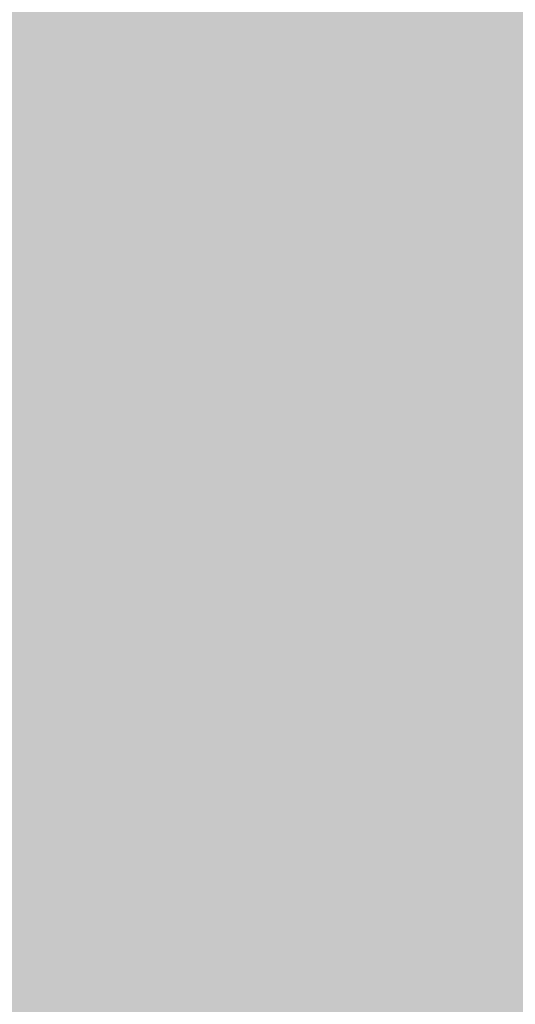
# Model space of a CAD drawing. Units: inches. Extents: x 2083 to 3317, y 1141 to 2115.
# Tile 165 of 256: x 3126.958245 to 3126.959398, y 1263.263648 to 1263.265937. Entities that reach past the tile are written whole.
import ezdxf

# ---------------------------------------------------------------- set-up
doc = ezdxf.new("R2010")
doc.units = ezdxf.units.IN
doc.layers.add('A-WALL-PATT', color=251, linetype='Continuous', lineweight=13, true_color=0x636466)

msp = doc.modelspace()

# ---------------------------------------------------------------- hatches: boundary and pattern name
at = {"layer": 'A-WALL-PATT'}
h = msp.add_hatch(color=256, dxfattribs=at)
h.dxf.hatch_style = 1
h.paths.add_polyline_path([(3126.9597832, 2020.7613601), (2748.9597832, 2020.7613601), (2604.9597832, 2020.7613601), (2226.9597832, 2020.7613601), (2226.9597832, 1702.7613601), (2466.9597832, 1702.7613601), (2466.9597832, 1582.7613601), (2418.9597832, 1582.7613601), (2418.9597832, 1477.7613601), (2226.9597832, 1477.7613601), (2226.9597832, 1263.2613601), (2544.9597832, 1263.2613601), (2544.9597832, 1411.7613601), (2604.9597832, 1411.7613601), (2685.9597832, 1411.7613601), (2685.9597832, 1420.7613601), (2604.9597832, 1420.7613601), (2604.9597832, 1573.7613601), (2604.9597832, 1702.7613601), (2604.9597832, 2011.7613601), (2748.9597832, 2011.7613601), (2748.9597832, 1702.7613601), (2862.9597832, 1702.7613601), (2862.9597832, 1621.7613601), (2871.9597832, 1621.7613601), (2871.9597832, 1702.7613601), (2883.9597832, 1702.7613601), (2883.9597832, 1706.9394595, -0.026459), (2883.9597832, 1711.7613601), (2757.9597832, 1711.7613601), (2757.9597832, 1807.7613601), (2787.9597832, 1807.7613601), (2787.9597832, 1812.2613601), (2757.9597832, 1812.2613601), (2757.9597832, 2011.7613601), (2877.9597832, 2011.7613601), (2877.9597832, 1812.2613601), (2847.9597832, 1812.2613601), (2847.9597832, 1807.7613601), (2889.8357425, 1807.7613601), (2889.8357425, 1812.2613601), (2882.4597832, 1812.2613601), (2882.4597832, 2011.7613601), (3117.9597832, 2011.7613601), (3117.9597832, 1812.2613601), (2937.8357425, 1812.2613601), (2937.8357425, 1807.7613601), (2995.7097832, 1807.7613601), (2995.7097832, 1796.1176655), (3000.2097832, 1796.1176655), (3000.2097832, 1807.7613601), (3117.9597832, 1807.7613601), (3117.9597832, 1711.7613601), (3000.2097832, 1711.7613601), (3000.2097832, 1760.1176655), (2998.5727047, 1760.1176655, -0.020711), (2995.7097832, 1760.1176655), (2995.7097832, 1711.7613601), (2931.9597832, 1711.7613601), (2931.9597832, 1702.7613601), (3126.9597832, 1702.7613601)])
h.paths.add_polyline_path([(2471.4597832, 2011.7613601), (2471.4597832, 1810.0113601), (2462.7169357, 1810.0113601), (2462.7169357, 1805.5113601), (2505.9597832, 1805.5113601), (2505.9597832, 1810.0113601), (2475.9597832, 1810.0113601), (2475.9597832, 2011.7613601), (2595.9597832, 2011.7613601), (2595.9597832, 1810.0113601), (2565.9597832, 1810.0113601), (2565.9597832, 1805.5113601), (2595.9597832, 1805.5113601), (2595.9597832, 1711.7613601), (2235.9597832, 1711.7613601), (2235.9597832, 1805.5113601), (2353.7097832, 1805.5113601), (2353.7097832, 1796.0541624), (2358.2097832, 1796.0541624), (2358.2097832, 1805.5113601), (2414.7169357, 1805.5113601), (2414.7169357, 1810.0113601), (2235.9597832, 1810.0113601), (2235.9597832, 2011.7613601)], flags=16)
h.paths.add_polyline_path([(2270.2047343, 1994.6100082), (2270.2047343, 1970.6100082), (2246.2047343, 1970.6100082), (2246.2047343, 1994.6100082)], flags=0)
edge = h.paths.add_edge_path(flags=0)
edge.add_ellipse((2332.027391, 1899.7981761), major_axis=(-3.0429938, 3.0429938), ratio=0.16825245, start_angle=-161.3321656, end_angle=-156.3071136, ccw=False)
edge.add_ellipse((2333.0820373, 1898.7435297), major_axis=(-1.0546463, 1.0546463), ratio=0.453532097, start_angle=-123.371019, end_angle=-94.1591066)
edge = h.paths.add_edge_path(flags=0)
edge.add_ellipse((2332.027391, 1968.8762897), major_axis=(3.0429938, 3.0429938), ratio=0.16825245, start_angle=18.6678344, end_angle=23.6928864)
edge.add_spline(control_points=[(2332.9255964, 1970.6911045), (2332.2267681, 1970.3360997), (2330.8937087, 1969.6589054), (2328.4130803, 1970.9321376), (2327.2039345, 1967.7487119), (2324.7095965, 1969.9555886), (2322.5328223, 1967.012354), (2320.0128462, 1971.2958124), (2317.6803077, 1968.1578449), (2316.0405263, 1967.1020468), (2315.4269045, 1966.8096022)], knot_values=[0, 0, 0, 0, 2.267059, 4.324559, 6.685584, 8.878641, 11.121502, 14.300359, 17.755284, 19.732645, 19.732645, 19.732645, 19.732645], degree=3, periodic=0)
edge.add_ellipse((2332.027391, 1968.8762897), major_axis=(3.0429938, 3.0429938), ratio=0.16825245, start_angle=18.6678344, end_angle=23.6928864, ccw=False)
edge.add_ellipse((2333.0820373, 1969.930936), major_axis=(1.0546463, 1.0546463), ratio=0.453532097, start_angle=56.628981, end_angle=85.8408934, ccw=False)
edge = h.paths.add_edge_path(flags=0)
edge.add_spline(control_points=[(2296.4282874, 1967.9879081), (2293.6278045, 1965.3363137), (2287.7036238, 1959.727094), (2299.7438601, 1949.9956993), (2294.5325909, 1935.6685275), (2290.5732281, 1920.6035119), (2293.3941244, 1909.9736911), (2296.1854073, 1904.9665431)], knot_values=[0.099185, 0.099185, 0.099185, 0.099185, 0.345301, 0.619822, 0.982653, 1.386093, 1.810555, 1.810555, 1.810555, 1.810555], degree=3, periodic=0)
edge.add_spline(control_points=[(2296.1854073, 1904.9665431), (2297.3835817, 1902.6193002), (2298.0009694, 1901.9493116), (2298.5529698, 1901.4681549)], knot_values=[0.006246, 0.006246, 0.006246, 0.006246, 0.055476, 0.055476, 0.055476, 0.055476], degree=3, periodic=0)
edge.add_spline(control_points=[(2298.5529698, 1901.4681549), (2297.2586121, 1900.9232238), (2295.2252939, 1900.2321257), (2293.0602287, 1900.6142053), (2292.1014227, 1900.788415), (2292.0895776, 1900.790568)], knot_values=[0.312835, 0.312835, 0.312835, 0.312835, 0.40178, 0.474987, 0.475903, 0.475903, 0.475903, 0.475903], degree=3, periodic=0)
edge.add_arc((2292.7936464, 1904.6641088), 3.9370079, 215.4208969, 259.6981795, ccw=False)
edge.add_spline(control_points=[(2289.5853139, 1902.3823039), (2289.4766524, 1902.5350874), (2289.3684805, 1902.6880353), (2289.2608648, 1902.8411699)], knot_values=[0.102872, 0.102872, 0.102872, 0.102872, 0.116896, 0.116896, 0.116896, 0.116896], degree=3, periodic=0)
edge.add_spline(control_points=[(2289.2608648, 1902.8411699), (2288.6866042, 1902.5501922), (2287.6400477, 1902.0199025), (2285.8813368, 1901.8739536), (2283.8529717, 1901.5043521), (2281.7199871, 1899.7105375), (2278.4669913, 1899.492942), (2276.1571361, 1901.8832022), (2272.2589526, 1899.8040711), (2267.7776054, 1901.8431828), (2262.2438819, 1900.1840326), (2257.414927, 1901.7820606), (2254.318374, 1900.7261196), (2253.1782849, 1900.3373431)], knot_values=[0, 0, 0, 0, 1.907977, 3.477176, 5.261074, 7.972851, 11.680248, 13.717921, 16.939592, 22.789562, 27.502503, 33.595215, 37.145618, 37.145618, 37.145618, 37.145618], degree=3, periodic=0)
edge.add_line((2253.1782849, 1900.3373431), (2250.2442397, 1902.8411699))
edge.add_line((2250.2442397, 1902.8411699), (2250.2442397, 1965.8332959))
edge.add_line((2250.2442397, 1965.8332959), (2253.1782849, 1968.3371226))
edge.add_spline(control_points=[(2253.1782849, 1968.3371226), (2254.318374, 1967.9483462), (2257.414927, 1966.8924051), (2262.2438819, 1968.4904332), (2267.7776054, 1966.8312829), (2271.5267301, 1968.5372172), (2273.8759143, 1967.8282895), (2274.2067012, 1967.7276424)], knot_values=[0, 0, 0, 0, 0.09018, 0.244935, 0.364644, 0.513233, 0.537855, 0.537855, 0.537855, 0.537855], degree=3, periodic=0)
edge.add_arc((2274.3528869, 1963.7933495), 3.9370079, 72.0511336, 92.1279492, ccw=False)
edge.add_arc((2281.2969331, 1985.2300027), 18.5962982, 252.05113361, 288.56572166)
edge.add_arc((2292.3167172, 1956.0288805), 12.6460805, 71.02678788, 113.77821843, ccw=False)
edge = h.paths.add_edge_path(flags=0)
edge.add_spline(control_points=[(2274.8994147, 1951.8561946), (2275.066156, 1951.6165924), (2275.2326866, 1951.3765878), (2275.3979871, 1951.1358545)], knot_values=[1.409916, 1.409916, 1.409916, 1.409916, 1.43159, 1.43159, 1.43159, 1.43159], degree=3, periodic=0)
edge.add_spline(control_points=[(2275.3979871, 1951.1358545), (2275.7921055, 1950.5618854), (2276.1792311, 1949.9837745), (2276.5455462, 1949.3971029)], knot_values=[1.358238, 1.358238, 1.358238, 1.358238, 1.409916, 1.409916, 1.409916, 1.409916], degree=3, periodic=0)
edge.add_line((2276.5455462, 1949.3971029), (2277.437289, 1947.8621847))
edge.add_spline(control_points=[(2277.437289, 1947.8621847), (2276.3038341, 1945.6731147), (2274.6396979, 1942.4268817), (2274.631615, 1938.0938998), (2272.7991237, 1930.8515498), (2274.3564261, 1943.8970461), (2275.9476814, 1947.9233558), (2276.5455462, 1949.3971029)], knot_values=[0.005632, 0.005632, 0.005632, 0.005632, 0.186014, 0.266002, 0.357087, 0.59639, 0.739732, 0.739732, 0.739732, 0.739732], degree=3, periodic=0)
edge.add_spline(control_points=[(2276.5455462, 1949.3971029), (2276.1792311, 1949.9837745), (2275.7921055, 1950.5618854), (2275.3979871, 1951.1358545)], knot_values=[1.358238, 1.358238, 1.358238, 1.358238, 1.409916, 1.409916, 1.409916, 1.409916], degree=3, periodic=0)
edge.add_spline(control_points=[(2275.3979871, 1951.1358545), (2274.9425002, 1950.0804523), (2274.2077604, 1948.0252718), (2273.9346018, 1944.8514774), (2272.4685341, 1937.6274891), (2273.4662155, 1945.6964663), (2274.7006154, 1951.0594725), (2274.8994147, 1951.8561946)], knot_values=[0.104364, 0.104364, 0.104364, 0.104364, 0.189636, 0.269624, 0.36071, 0.600013, 0.644622, 0.644622, 0.644622, 0.644622], degree=3, periodic=0)
h.paths.add_polyline_path([(2269.1675139, 1963.1275729, -0.357527), (2268.170633, 1960.9763695, -0.092561), (2268.170633, 1939.4363249, -0.357527), (2269.1675139, 1937.2851215, -0.357527), (2267.0163105, 1938.2820024, -0.164785), (2254.6855813, 1938.2820024, -0.357527), (2252.5343779, 1937.2851215, -0.357527), (2253.5312587, 1939.4363249, -0.092561), (2253.5312587, 1960.9763695, -0.357527), (2252.5343779, 1963.1275729, -0.357527), (2254.6855813, 1962.130692, -0.164785), (2267.0163105, 1962.130692, -0.357527)], flags=0)
h.paths.add_polyline_path([(2248.8740679, 1967.8017998), (2248.8740679, 1957.0277095), (2249.4577833, 1957.0277095), (2249.4577833, 1911.6467562), (2248.8740679, 1911.6467562), (2248.8740679, 1900.8726659), (2246.5118632, 1900.8726659, 0.197327), (2244.1496584, 1902.4568734), (2244.1496584, 1966.2175923, 0.197327), (2246.5118632, 1967.8017998)], flags=0)
h.paths.add_polyline_path([(2269.1675139, 1931.3893442, -0.357527), (2268.170633, 1929.2381408, -0.092561), (2268.170633, 1907.6980962, -0.357527), (2269.1675139, 1905.5468928, -0.357527), (2267.0163105, 1906.5437737, -0.164785), (2254.6855813, 1906.5437737, -0.357527), (2252.5343779, 1905.5468928, -0.357527), (2253.5312587, 1907.6980962, -0.092561), (2253.5312587, 1929.2381408, -0.357527), (2252.5343779, 1931.3893442, -0.357527), (2254.6855813, 1930.3924634, -0.164785), (2267.0163105, 1930.3924634, -0.357527)], flags=0)
edge = h.paths.add_edge_path(flags=0)
edge.add_spline(control_points=[(2276.1968578, 1906.7237016), (2276.1681442, 1909.0289278), (2276.1140492, 1913.371852), (2270.5984171, 1924.9249783), (2273.9051746, 1919.0127787), (2275.9217115, 1916.2620626), (2275.4745699, 1912.4021495), (2277.2578735, 1910.3806206), (2276.6960436, 1908.2250358), (2276.6462176, 1906.8130226), (2276.6178249, 1906.0084068)], knot_values=[0, 0, 0, 0, 8.61026, 16.221274, 18.843057, 23.804898, 27.440828, 29.356102, 31.203478, 33.650687, 33.650687, 33.650687, 33.650687], degree=3, periodic=0)
edge.add_spline(control_points=[(2276.6178249, 1906.0084068), (2276.6233131, 1905.6241436), (2276.4977381, 1904.6286608), (2275.4417789, 1903.8547251), (2274.9373144, 1903.0804497), (2274.8590804, 1902.8411699)], knot_values=[0.156488, 0.156488, 0.156488, 0.156488, 0.184398, 0.231376, 0.250598, 0.250598, 0.250598, 0.250598], degree=3, periodic=0)
edge.add_line((2274.8590804, 1902.8411699), (2276.50598, 1902.8411699))
edge.add_spline(control_points=[(2276.50598, 1902.8411699), (2276.7883084, 1903.0849395), (2277.6650711, 1904.1251958), (2278.2495378, 1904.340738), (2277.6538719, 1908.5273866), (2278.15567, 1906.2278078), (2278.100464, 1905.2859484), (2278.8466748, 1904.0690054), (2277.8567853, 1903.4149482), (2277.8741909, 1902.9910497), (2277.9035616, 1902.8411699)], knot_values=[0.059574, 0.059574, 0.059574, 0.059574, 0.080753, 0.103741, 0.16972, 0.176036, 0.207137, 0.240474, 0.262341, 0.27366, 0.27366, 0.27366, 0.27366], degree=3, periodic=0)
edge.add_line((2277.9035616, 1902.8411699), (2280.0298255, 1902.8411699))
edge.add_spline(control_points=[(2280.0298255, 1902.8411699), (2279.8882214, 1903.088398), (2279.4992571, 1903.9815512), (2280.1522839, 1905.9393491), (2278.103615, 1909.6577572), (2279.7623946, 1907.185285), (2280.3279002, 1904.8748608), (2280.4851086, 1903.4895904), (2281.4632687, 1903.2494323), (2281.7583431, 1902.9364967), (2281.8340361, 1902.8411699)], knot_values=[0.013856, 0.013856, 0.013856, 0.013856, 0.034874, 0.088867, 0.107879, 0.126738, 0.158714, 0.193757, 0.217487, 0.226722, 0.226722, 0.226722, 0.226722], degree=3, periodic=0)
edge.add_spline(control_points=[(2281.8340361, 1902.8411699), (2281.7875348, 1902.8267029), (2281.6470224, 1902.7829881), (2281.3955272, 1902.85949), (2281.088077, 1902.9852418), (2280.7206826, 1903.060902), (2280.3334513, 1903.0257257), (2280.1247668, 1902.898879), (2280.0298255, 1902.8411699)], knot_values=[0, 0, 0, 0, 0.14413, 0.435517, 0.749276, 1.153046, 1.548371, 1.878348, 1.878348, 1.878348, 1.878348], degree=3, periodic=0)
edge.add_line((2280.0298255, 1902.8411699), (2277.9035616, 1902.8411699))
edge.add_spline(control_points=[(2277.9035616, 1902.8411699), (2277.892855, 1902.7958553), (2277.865396, 1902.6796374), (2277.6074793, 1902.6874828), (2277.2740503, 1902.8006999), (2276.8379209, 1902.6197745), (2276.5838074, 1902.7892611), (2276.50598, 1902.8411699)], knot_values=[0, 0, 0, 0, 0.127189, 0.326199, 0.628009, 1.24357, 1.515331, 1.515331, 1.515331, 1.515331], degree=3, periodic=0)
edge.add_line((2276.50598, 1902.8411699), (2274.8590804, 1902.8411699))
edge.add_spline(control_points=[(2274.8590804, 1902.8411699), (2274.8144367, 1902.8985868), (2274.7251297, 1903.013446), (2274.4934765, 1903.1189684), (2274.2442854, 1902.9605386), (2273.9371207, 1903.1849416), (2273.6140395, 1902.9831428), (2273.4083164, 1902.8830449), (2273.322254, 1902.8411699)], knot_values=[0, 0, 0, 0, 0.21843, 0.436957, 0.687977, 0.990379, 1.398396, 1.69185, 1.69185, 1.69185, 1.69185], degree=3, periodic=0)
edge.add_spline(control_points=[(2273.322254, 1902.8411699), (2273.6167403, 1903.445692), (2274.2739977, 1904.5382529), (2276.0272387, 1904.5737017), (2276.2069634, 1906.5836372), (2276.1968578, 1906.7237016)], knot_values=[0.012227, 0.012227, 0.012227, 0.012227, 0.059472, 0.106218, 0.134458, 0.134458, 0.134458, 0.134458], degree=3, periodic=0)
h.paths.add_polyline_path([(2270.7760538, 1897.7898284), (2270.7760538, 1873.7898284), (2246.7760538, 1873.7898284), (2246.7760538, 1897.7898284)], flags=0)
h.paths.add_polyline_path([(2353.7097832, 1760.0050593), (2353.7097832, 1760.0541624), (2358.2097832, 1760.0541624, -0.033729)], flags=0)
h.paths.add_polyline_path([(2321.8191188, 1737.5291862), (2341.9953271, 1737.5291862, -0.414214), (2343.2032727, 1736.3212406), (2343.2032727, 1721.0205964, -0.414214), (2341.9953271, 1719.8126508), (2321.8191188, 1719.8126508, -0.414214), (2320.6111732, 1721.0205964), (2320.6111732, 1736.3212406, -0.414214)], flags=0)
h.paths.add_polyline_path([(2324.2350099, 1736.3212406), (2339.5794359, 1736.3212406, -0.414214), (2341.9953271, 1733.9053494), (2341.9953271, 1725.4497302, -0.414214), (2339.5794359, 1723.033839), (2333.6805885, 1723.033839), (2333.8453172, 1722.0454666, -0.870646), (2335.4253988, 1721.8258934, -0.767327), (2333.922694, 1721.4232449), (2331.2910241, 1721.4232449, -0.767327), (2329.7883193, 1721.8258934, -0.870646), (2331.3684009, 1722.0454666), (2331.5331296, 1723.033839), (2324.2350099, 1723.033839, -0.414214), (2321.8191188, 1725.4497302), (2321.8191188, 1733.9053494, -0.414214)], flags=0)
h.paths.add_polyline_path([(2570.4837892, 1928.6154443), (2589.6837892, 1928.6154443), (2590.1688286, 1928.6154443), (2590.1688286, 1904.9933971), (2570.4837892, 1904.9933971)], flags=0)
h.paths.add_polyline_path([(2574.4473242, 1927.2638215, -1), (2572.8288357, 1927.2638215, -1)], flags=0)
h.paths.add_polyline_path([(2573.0898665, 1926.9408768), (2573.925032, 1927.7760423), (2574.1477428, 1927.5533315), (2573.3125773, 1926.718166)], flags=0)
h.paths.add_polyline_path([(2578.7790648, 1919.7296175, -1), (2571.5916632, 1919.7296175, -1)], flags=0)
h.paths.add_polyline_path([(2578.385364, 1919.7296175, -1), (2571.985364, 1919.7296175, -1)], flags=0)
h.paths.add_polyline_path([(2331.5957638, 1729.4762156, -1), (2333.6179542, 1729.4762156, -1)], flags=0)
h.paths.add_polyline_path([(2578.0342282, 1927.2638215, -1), (2576.4157396, 1927.2638215, -1)], flags=0)
h.paths.add_polyline_path([(2576.6888513, 1927.5310886), (2576.9115621, 1927.7537993), (2577.7467276, 1926.9186339), (2577.5240168, 1926.6959231)], flags=0)
h.paths.add_polyline_path([(2578.1390648, 1909.8595388, -1), (2572.2316632, 1909.8595388, -1)], flags=0)
h.paths.add_polyline_path([(2577.745364, 1909.8595388, -1), (2572.625364, 1909.8595388, -1)], flags=0)
h.paths.add_polyline_path([(2583.7977179, 1927.2638215, -1), (2582.1792294, 1927.2638215, -1)], flags=0)
h.paths.add_polyline_path([(2582.7186487, 1927.7537993), (2583.5538142, 1926.9186339), (2583.3311034, 1926.6959231), (2582.4959379, 1927.5310886)], flags=0)
h.paths.add_polyline_path([(2582.4959379, 1927.5310886), (2582.7186487, 1927.7537993), (2583.5538142, 1926.9186339), (2583.3311034, 1926.6959231)], flags=0)
h.paths.add_polyline_path([(2587.7390648, 1920.5296175, -1), (2581.8316632, 1920.5296175, -1)], flags=0)
h.paths.add_polyline_path([(2587.345364, 1920.5296175, -1), (2582.225364, 1920.5296175, -1)], flags=0)
h.paths.add_polyline_path([(2587.3846219, 1927.2638215, -1), (2585.7661333, 1927.2638215, -1)], flags=0)
h.paths.add_polyline_path([(2586.0819925, 1926.9802469), (2586.917158, 1927.8154124), (2587.1398688, 1927.5927016), (2586.3047033, 1926.7575361)], flags=0)
h.paths.add_polyline_path([(2588.3790648, 1910.6595388, -1), (2581.1916632, 1910.6595388, -1)], flags=0)
h.paths.add_polyline_path([(2587.985364, 1910.6595388, -1), (2581.585364, 1910.6595388, -1)], flags=0)
h.paths.add_polyline_path([(2417.1677288, 1729.4778955), (2437.3439372, 1729.4778955, -0.414214), (2438.5518828, 1728.2699499), (2438.5518828, 1712.9693057, -0.414214), (2437.3439372, 1711.7613601), (2417.1677288, 1711.7613601, -0.414214), (2415.9597832, 1712.9693057), (2415.9597832, 1728.2699499, -0.414214)], flags=0)
h.paths.add_polyline_path([(2419.58362, 1728.2699499), (2434.928046, 1728.2699499, -0.414214), (2437.3439372, 1725.8540587), (2437.3439372, 1717.3984395, -0.414214), (2434.928046, 1714.9825483), (2429.0291985, 1714.9825483), (2429.1939273, 1713.9941758, -0.870646), (2430.7740089, 1713.7746027, -0.767327), (2429.2713041, 1713.3719542), (2426.6396342, 1713.3719542, -0.767327), (2425.1369294, 1713.7746027, -0.870646), (2426.717011, 1713.9941758), (2426.8817397, 1714.9825483), (2419.58362, 1714.9825483, -0.414214), (2417.1677288, 1717.3984395), (2417.1677288, 1725.8540587, -0.414214)], flags=0)
h.paths.add_polyline_path([(2419.58362, 1728.2699499), (2434.928046, 1728.2699499, -0.414214), (2437.3439372, 1725.8540587), (2437.3439372, 1717.3984395, -0.414214), (2434.928046, 1714.9825483), (2429.0291985, 1714.9825483), (2428.3581177, 1719.0090337), (2427.5528206, 1719.0090337), (2426.8817397, 1714.9825483), (2419.58362, 1714.9825483, -0.414214), (2417.1677288, 1717.3984395), (2417.1677288, 1725.8540587, -0.414214)], flags=0)
h.paths.add_polyline_path([(2426.9443739, 1721.4249248, -1), (2428.9665643, 1721.4249248, -1)], flags=0)
h.paths.add_polyline_path([(2475.9597832, 1702.7613601), (2595.9597832, 1702.7613601), (2595.9597832, 1582.7613601), (2475.9597832, 1582.7613601)], flags=16)
h.paths.add_polyline_path([(2427.9597832, 1573.7613601), (2595.9597832, 1573.7613601), (2595.9597832, 1468.7613601), (2595.9597832, 1420.7613601), (2384.4597832, 1420.7613601), (2384.4597832, 1468.7613601), (2427.9597832, 1468.7613601)], flags=16)
h.paths.add_polyline_path([(2379.9597832, 1468.7613601), (2379.9597832, 1420.7613601), (2235.9597832, 1420.7613601), (2235.9597832, 1468.7613601)], flags=16)
h.paths.add_polyline_path([(2317.8159962, 1466.695767), (2337.9922045, 1466.695767, -0.414214), (2339.2001501, 1465.4878214), (2339.2001501, 1450.1871771, -0.414214), (2337.9922045, 1448.9792315), (2317.8159962, 1448.9792315, -0.414214), (2316.6080506, 1450.1871771), (2316.6080506, 1465.4878214, -0.414214)], flags=0)
h.paths.add_polyline_path([(2320.2318874, 1465.4878214), (2335.5763133, 1465.4878214, -0.414214), (2337.9922045, 1463.0719302), (2337.9922045, 1454.616311, -0.414214), (2335.5763133, 1452.2004198), (2329.6774659, 1452.2004198), (2329.8421946, 1451.2120473, -0.870646), (2331.4222762, 1450.9924742, -0.767327), (2329.9195714, 1450.5898257), (2327.2879015, 1450.5898257, -0.767327), (2325.7851967, 1450.9924742, -0.870646), (2327.3652783, 1451.2120473), (2327.530007, 1452.2004198), (2320.2318874, 1452.2004198, -0.414214), (2317.8159962, 1454.616311), (2317.8159962, 1463.0719302, -0.414214)], flags=0)
h.paths.add_polyline_path([(2320.2318874, 1465.4878214), (2335.5763133, 1465.4878214, -0.414214), (2337.9922045, 1463.0719302), (2337.9922045, 1454.616311, -0.414214), (2335.5763133, 1452.2004198), (2329.6774659, 1452.2004198), (2329.006385, 1456.2269051), (2328.2010879, 1456.2269051), (2327.530007, 1452.2004198), (2320.2318874, 1452.2004198, -0.414214), (2317.8159962, 1454.616311), (2317.8159962, 1463.0719302, -0.414214)], flags=0)
h.paths.add_polyline_path([(2327.5926413, 1458.6427963, -1), (2329.6148317, 1458.6427963, -1)], flags=0)
h.paths.add_polyline_path([(2244.4117436, 1433.3404531), (2241.9209449, 1433.3404531, -0.414214), (2240.0178562, 1435.2435418), (2240.0178562, 1440.9528078, -0.414211), (2241.920925, 1442.8558965), (2244.4117436, 1442.8558965, -1.976472)], flags=0)
h.paths.add_polyline_path([(2245.3568884, 1434.3975358, -0.414214), (2245.3568884, 1441.7988138, -2.144098)], flags=0)
h.paths.add_polyline_path([(2535.9597832, 1416.2613601), (2535.9597832, 1272.2613601), (2235.9597832, 1272.2613601), (2235.9597832, 1416.2613601)], flags=16)
h.paths.add_polyline_path([(2260.1195614, 1384.2928413), (2260.1195614, 1362.0386487), (2237.8653688, 1362.0386487), (2237.8653688, 1384.2928413)], flags=0)
edge = h.paths.add_edge_path(flags=0)
edge.add_line((2318.2518466, 1362.0932983), (2318.1457968, 1362.0009726))
edge.add_ellipse((2317.4451158, 1360.4310442), major_axis=(2.8216404, 2.8216404), ratio=0.16825245, start_angle=18.6678344, end_angle=20.9481273, ccw=False)
edge.add_ellipse((2318.4230451, 1361.4089735), major_axis=(0.9779293, 0.9779293), ratio=0.453532097, start_angle=56.628981, end_angle=70.2262012, ccw=False)
edge = h.paths.add_edge_path(flags=0)
edge.add_line((2319.1073699, 1295.5710784), (2319.0150442, 1295.6771282))
edge.add_ellipse((2317.4451158, 1296.3778091), major_axis=(-2.8216404, 2.8216404), ratio=0.16825245, start_angle=-161.3321656, end_angle=-159.0518727, ccw=False)
edge.add_ellipse((2318.4230451, 1295.3998798), major_axis=(-0.9779293, 0.9779293), ratio=0.453532097, start_angle=-123.371019, end_angle=-109.7737988)
edge = h.paths.add_edge_path(flags=0)
edge.add_spline(control_points=[(2284.2103489, 1301.1702189), (2284.5806878, 1300.444719), (2284.8911891, 1299.8920243), (2285.159553, 1299.4610182)], knot_values=[0.039066, 0.039066, 0.039066, 0.039066, 0.055476, 0.055476, 0.055476, 0.055476], degree=3, periodic=0)
edge.add_line((2285.159553, 1299.4610182), (2284.2103489, 1301.1702189))
edge = h.paths.add_edge_path(flags=0)
edge.add_line((2280.4124579, 1297.2980125), (2283.3699905, 1297.0361216))
edge.add_line((2283.3699905, 1297.0361216), (2286.4056902, 1297.9263104))
edge.add_spline(control_points=[(2286.4056902, 1297.9263104), (2285.305487, 1297.4631193), (2284.3447774, 1297.1291508), (2283.3699905, 1297.0361216)], knot_values=[0.394369, 0.394369, 0.394369, 0.394369, 0.475903, 0.475903, 0.475903, 0.475903], degree=3, periodic=0)
edge.add_spline(control_points=[(2283.3699905, 1297.0361216), (2283.2813895, 1297.027666), (2282.316289, 1296.9573356), (2281.3125019, 1297.1344787), (2280.4234414, 1297.2960161), (2280.4124579, 1297.2980125)], knot_values=[0.312835, 0.312835, 0.312835, 0.312835, 0.320246, 0.393453, 0.394369, 0.394369, 0.394369, 0.394369], degree=3, periodic=0)
edge = h.paths.add_edge_path(flags=0)
edge.add_line((2284.4355615, 1359.6072854), (2280.4462909, 1355.328047))
edge.add_line((2280.4462909, 1355.328047), (2279.5799868, 1351.0177544))
edge.add_line((2279.5799868, 1351.0177544), (2282.4129737, 1346.5804327))
edge.add_spline(control_points=[(2282.4129737, 1346.5804327), (2283.1533308, 1345.5892358), (2284.2528957, 1344.0288973), (2284.801037, 1342.3871671), (2284.9351625, 1341.8055443)], knot_values=[1.240098, 1.240098, 1.240098, 1.240098, 1.332892, 1.382712, 1.382712, 1.382712, 1.382712], degree=3, periodic=0)
edge.add_spline(control_points=[(2284.9351625, 1341.8055443), (2285.3191079, 1340.1406002), (2285.2330291, 1338.4092041), (2284.9099384, 1336.6541222)], knot_values=[1.097484, 1.097484, 1.097484, 1.097484, 1.240098, 1.240098, 1.240098, 1.240098], degree=3, periodic=0)
edge.add_spline(control_points=[(2284.9099384, 1336.6541222), (2284.5868478, 1334.8990403), (2284.0267453, 1333.1202725), (2283.4626437, 1331.3605849)], knot_values=[0.95487, 0.95487, 0.95487, 0.95487, 1.097484, 1.097484, 1.097484, 1.097484], degree=3, periodic=0)
edge.add_line((2283.4626437, 1331.3605849), (2281.8903759, 1326.153357))
edge.add_line((2281.8903759, 1326.153357), (2280.7562592, 1321.0560888))
edge.add_line((2280.7562592, 1321.0560888), (2280.2992048, 1316.0019772))
edge.add_line((2280.2992048, 1316.0019772), (2280.7159327, 1310.9500678))
edge.add_line((2280.7159327, 1310.9500678), (2282.0280939, 1305.9721367))
edge.add_line((2282.0280939, 1305.9721367), (2284.2103489, 1301.1702189))
edge.add_spline(control_points=[(2284.2103489, 1301.1702189), (2283.3407305, 1302.7301854), (2282.6119044, 1304.3364933), (2282.0280939, 1305.9721367)], knot_values=[0.099185, 0.099185, 0.099185, 0.099185, 0.241799, 0.241799, 0.241799, 0.241799], degree=3, periodic=0)
edge.add_spline(control_points=[(2282.0280939, 1305.9721367), (2281.4442835, 1307.6077801), (2281.0054886, 1309.2727591), (2280.7159327, 1310.9500678)], knot_values=[0.241799, 0.241799, 0.241799, 0.241799, 0.384413, 0.384413, 0.384413, 0.384413], degree=3, periodic=0)
edge.add_spline(control_points=[(2280.7159327, 1310.9500678), (2280.4332411, 1312.5876134), (2280.2893863, 1314.2769594), (2280.2988938, 1315.9620324), (2280.2992048, 1316.0019772)], knot_values=[0.384413, 0.384413, 0.384413, 0.384413, 0.523647, 0.527028, 0.527028, 0.527028, 0.527028], degree=3, periodic=0)
edge.add_spline(control_points=[(2280.2992048, 1316.0019772), (2280.3123257, 1317.6869552), (2280.4778706, 1319.3679256), (2280.7562592, 1321.0560888)], knot_values=[0.527028, 0.527028, 0.527028, 0.527028, 0.669642, 0.669642, 0.669642, 0.669642], degree=3, periodic=0)
edge.add_spline(control_points=[(2280.7562592, 1321.0560888), (2281.0346478, 1322.7442519), (2281.4258801, 1324.4396079), (2281.8903759, 1326.153357)], knot_values=[0.669642, 0.669642, 0.669642, 0.669642, 0.812256, 0.812256, 0.812256, 0.812256], degree=3, periodic=0)
edge.add_spline(control_points=[(2281.8903759, 1326.153357), (2282.2643834, 1327.5332507), (2282.7878702, 1329.2618097), (2283.352751, 1331.0177803), (2283.4626437, 1331.3605849)], knot_values=[0.812256, 0.812256, 0.812256, 0.812256, 0.927087, 0.95487, 0.95487, 0.95487, 0.95487], degree=3, periodic=0)
edge.add_line((2283.4626437, 1331.3605849), (2284.9099384, 1336.6541222))
edge.add_line((2284.9099384, 1336.6541222), (2284.9351625, 1341.8055443))
edge.add_line((2284.9351625, 1341.8055443), (2282.4129737, 1346.5804327))
edge.add_spline(control_points=[(2282.4129737, 1346.5804327), (2281.2751273, 1348.1037918), (2280.0784467, 1349.5703178), (2279.5799868, 1351.0177544)], knot_values=[1.382712, 1.382712, 1.382712, 1.382712, 1.525326, 1.525326, 1.525326, 1.525326], degree=3, periodic=0)
edge.add_spline(control_points=[(2279.5799868, 1351.0177544), (2279.4432818, 1351.4147209), (2279.1363124, 1352.856922), (2279.7351897, 1354.2903851), (2280.4462909, 1355.328047)], knot_values=[1.525326, 1.525326, 1.525326, 1.525326, 1.564439, 1.667941, 1.667941, 1.667941, 1.667941], degree=3, periodic=0)
edge.add_spline(control_points=[(2280.4462909, 1355.328047), (2281.4261132, 1356.7578354), (2282.9308373, 1358.1825604), (2284.4355615, 1359.6072854)], knot_values=[1.667941, 1.667941, 1.667941, 1.667941, 1.810555, 1.810555, 1.810555, 1.810555], degree=3, periodic=0)
edge.add_arc((2280.6230749, 1348.518181), 11.7261796, 71.02678788, 113.77821843)
edge.add_arc((2270.4048917, 1375.5951559), 17.2435667, 252.05113361, 288.56572166, ccw=False)
edge.add_arc((2263.9659692, 1355.7178471), 3.6506221, 72.0511336, 92.1279492)
edge.add_arc((2263.9659692, 1355.7178471), 3.6506221, 92.1279492, 177.98513)
edge.add_spline(control_points=[(2260.3176041, 1355.8461989), (2260.2604169, 1354.2206683), (2260.551278, 1350.1865469), (2262.9993445, 1346.7662507), (2264.4727415, 1344.6490245)], knot_values=[1.43159, 1.43159, 1.43159, 1.43159, 1.564144, 1.770695, 1.770695, 1.770695, 1.770695], degree=3, periodic=0)
edge.add_line((2264.4727415, 1344.6490245), (2264.9355904, 1343.9825301))
edge.add_spline(control_points=[(2263.8010444, 1340.2481052), (2263.8432379, 1340.5140884), (2264.0672444, 1341.7564652), (2264.5126928, 1343.0024532), (2264.9350468, 1343.9810834)], knot_values=[0.53657, 0.53657, 0.53657, 0.53657, 0.559349, 0.644622, 0.644622, 0.644622, 0.644622], degree=3, periodic=0)
edge.add_spline(control_points=[(2264.9350468, 1343.9810834), (2265.1177715, 1343.7149747), (2265.2988751, 1343.4479058), (2265.4767562, 1343.1793646)], knot_values=[1.384077, 1.384077, 1.384077, 1.384077, 1.409916, 1.409916, 1.409916, 1.409916], degree=3, periodic=0)
edge.add_spline(control_points=[(2265.4767562, 1343.1793646), (2265.6546373, 1342.9108234), (2265.8292958, 1342.64081), (2265.9991301, 1342.368812)], knot_values=[1.358238, 1.358238, 1.358238, 1.358238, 1.384077, 1.384077, 1.384077, 1.384077], degree=3, periodic=0)
edge.add_line((2265.9991301, 1342.368812), (2266.8260057, 1340.9455468))
edge.add_spline(control_points=[(2266.8260057, 1340.9455468), (2268.894401, 1337.0896912), (2271.3981727, 1325.8430009), (2270.5161644, 1310.5685568), (2275.9193759, 1301.860609), (2277.7895113, 1299.1994495)], knot_values=[0.116896, 0.116896, 0.116896, 0.116896, 0.472987, 1.050969, 1.313793, 1.313793, 1.313793, 1.313793], degree=3, periodic=0)
edge.add_spline(control_points=[(2277.7895113, 1299.1994495), (2277.8394051, 1299.1284519), (2277.8894277, 1299.0574975), (2277.9395717, 1298.9865839)], knot_values=[0.109884, 0.109884, 0.109884, 0.109884, 0.116896, 0.116896, 0.116896, 0.116896], degree=3, periodic=0)
edge.add_line((2277.9395717, 1298.9865839), (2277.7888489, 1299.1991139))
edge.add_spline(control_points=[(2277.7888489, 1299.1991139), (2277.2565819, 1298.9294144), (2276.2863504, 1298.4379024), (2275.0393517, 1298.3344186), (2274.3833299, 1298.2388951), (2274.2152543, 1298.209338)], knot_values=[33.12187, 33.12187, 33.12187, 33.12187, 35.029056, 36.598255, 37.144827, 37.144827, 37.144827, 37.144827], degree=3, periodic=0)
edge.add_line((2274.2152543, 1298.209338), (2273.073147, 1297.8929607))
edge.add_spline(control_points=[(2273.073147, 1297.8929607), (2272.3229363, 1297.579784), (2271.0391507, 1296.5105078), (2269.2483948, 1296.2260622), (2268.4231004, 1296.3746543)], knot_values=[26.532584, 26.532584, 26.532584, 26.532584, 29.198919, 31.839101, 31.839101, 31.839101, 31.839101], degree=3, periodic=0)
edge.add_line((2268.4231004, 1296.3746543), (2263.8785014, 1297.4575338))
edge.add_spline(control_points=[(2263.8785014, 1297.4575338), (2263.5560769, 1297.3594345), (2261.8603064, 1296.8386943), (2260.2387805, 1297.2824073), (2258.9334543, 1297.5164611)], knot_values=[15.919551, 15.919551, 15.919551, 15.919551, 16.939592, 21.226067, 21.226067, 21.226067, 21.226067], degree=3, periodic=0)
edge.add_line((2258.9334543, 1297.5164611), (2254.0552332, 1297.3290098))
edge.add_spline(control_points=[(2254.0552332, 1297.3290098), (2253.7555255, 1297.295815), (2252.1136834, 1297.1651738), (2250.4618687, 1297.5442209), (2249.1296862, 1297.6678818)], knot_values=[5.306517, 5.306517, 5.306517, 5.306517, 6.276435, 10.613034, 10.613034, 10.613034, 10.613034], degree=3, periodic=0)
edge.add_line((2249.1296862, 1297.6678818), (2244.3316495, 1296.8777561))
edge.add_line((2244.3316495, 1296.8777561), (2241.6110326, 1299.1994495))
edge.add_line((2241.6110326, 1299.1994495), (2241.6110326, 1357.6094038))
edge.add_line((2241.6110326, 1357.6094038), (2244.3316495, 1359.9310973))
edge.add_line((2244.3316495, 1359.9310973), (2252.7288228, 1359.5426917))
edge.add_spline(control_points=[(2252.7288228, 1359.5426917), (2252.8709387, 1359.5464396), (2253.3057402, 1359.5481716), (2253.7398447, 1359.5142744), (2254.0317419, 1359.4824261)], knot_values=[0.233291, 0.233291, 0.233291, 0.233291, 0.244935, 0.268927, 0.268927, 0.268927, 0.268927], degree=3, periodic=0)
edge.add_line((2254.0317419, 1359.4824261), (2259.5871899, 1359.4163899))
edge.add_spline(control_points=[(2259.5871899, 1359.4163899), (2260.6770676, 1359.6285026), (2262.0731971, 1359.8970025), (2263.5236925, 1359.4592776), (2263.8304173, 1359.3659518)], knot_values=[0.422516, 0.422516, 0.422516, 0.422516, 0.513233, 0.537855, 0.537855, 0.537855, 0.537855], degree=3, periodic=0)
edge.add_arc((2263.9659692, 1355.7178471), 3.6506221, 72.0511336, 92.1279492, ccw=False)
edge.add_arc((2270.4048917, 1375.5951559), 17.2435667, 252.05113361, 288.56572166)
edge.add_arc((2280.6230749, 1348.518181), 11.7261796, 71.02678788, 113.77821843, ccw=False)
h.paths.add_polyline_path([(2240.3405298, 1359.4347149), (2240.3405298, 1349.4443532), (2240.8817846, 1349.4443532), (2240.8817846, 1307.3645001), (2240.3405298, 1307.3645001), (2240.3405298, 1297.3741385), (2238.1501565, 1297.3741385, 0.197327), (2235.9597832, 1298.8431076), (2235.9597832, 1357.9657458, 0.197327), (2238.1501565, 1359.4347149)], flags=0)
h.paths.add_polyline_path([(2259.1577904, 1355.1005005, -0.357527), (2258.2334246, 1353.1057799, -0.092561), (2258.2334246, 1333.1326007, -0.357527), (2259.1577904, 1331.1378801, -0.357527), (2257.1630698, 1332.0622458, -0.164785), (2245.7293022, 1332.0622458, -0.357527), (2243.7345816, 1331.1378801, -0.357527), (2244.6589474, 1333.1326007, -0.092561), (2244.6589474, 1353.1057799, -0.357527), (2243.7345816, 1355.1005005, -0.357527), (2245.7293022, 1354.1761347, -0.164785), (2257.1630698, 1354.1761347, -0.357527)], flags=0)
edge = h.paths.add_edge_path(flags=0)
edge.add_line((2265.9991301, 1342.368812), (2266.8260057, 1340.9455468))
edge.add_line((2266.8260057, 1340.9455468), (2265.3075567, 1337.8140664))
edge.add_line((2265.3075567, 1337.8140664), (2264.358232, 1334.6529388))
edge.add_line((2264.358232, 1334.6529388), (2264.2620123, 1333.7997046))
edge.add_spline(control_points=[(2264.2620123, 1333.7997046), (2264.2083565, 1333.187055), (2264.1620602, 1332.3655252), (2264.0071444, 1331.4139326), (2263.9690487, 1331.2018338)], knot_values=[0.464444, 0.464444, 0.464444, 0.464444, 0.516691, 0.531608, 0.531608, 0.531608, 0.531608], degree=3, periodic=0)
edge.add_spline(control_points=[(2263.9690487, 1331.2018338), (2263.7745349, 1330.1188727), (2263.4243703, 1328.7908386), (2263.2574202, 1328.5306516), (2263.2340282, 1328.5146115)], knot_values=[0.372682, 0.372682, 0.372682, 0.372682, 0.44885, 0.464444, 0.464444, 0.464444, 0.464444], degree=3, periodic=0)
edge.add_spline(control_points=[(2263.2340282, 1328.5146115), (2263.096382, 1328.4202271), (2263.1311696, 1329.3014765), (2263.2749528, 1330.6157493)], knot_values=[0.280919, 0.280919, 0.280919, 0.280919, 0.372682, 0.372682, 0.372682, 0.372682], degree=3, periodic=0)
edge.add_spline(control_points=[(2263.2749528, 1330.6157493), (2263.4187361, 1331.930022), (2263.6715151, 1333.677318), (2263.9698519, 1335.3150268)], knot_values=[0.189157, 0.189157, 0.189157, 0.189157, 0.280919, 0.280919, 0.280919, 0.280919], degree=3, periodic=0)
edge.add_spline(control_points=[(2263.9698519, 1335.3150268), (2264.1004958, 1336.0321917), (2264.4187827, 1337.6219113), (2264.7548476, 1338.8644304), (2264.9474193, 1339.4911244)], knot_values=[0.097394, 0.097394, 0.097394, 0.097394, 0.137578, 0.189157, 0.189157, 0.189157, 0.189157], degree=3, periodic=0)
edge.add_spline(control_points=[(2264.9474193, 1339.4911244), (2265.2900171, 1340.6060546), (2265.6442376, 1341.4939958), (2265.9991301, 1342.368812)], knot_values=[0.005632, 0.005632, 0.005632, 0.005632, 0.097394, 0.097394, 0.097394, 0.097394], degree=3, periodic=0)
h.paths.add_polyline_path([(2259.1577904, 1325.6709733, -0.357527), (2258.2334246, 1323.6762527, -0.092561), (2258.2334246, 1303.7030735, -0.357527), (2259.1577904, 1301.7083529, -0.357527), (2257.1630698, 1302.6327186, -0.164785), (2245.7293022, 1302.6327186, -0.357527), (2243.7345816, 1301.7083529, -0.357527), (2244.6589474, 1303.7030735, -0.092561), (2244.6589474, 1323.6762527, -0.357527), (2243.7345816, 1325.6709733, -0.357527), (2245.7293022, 1324.7466075, -0.164785), (2257.1630698, 1324.7466075, -0.357527)], flags=0)
edge = h.paths.add_edge_path(flags=0)
edge.add_spline(control_points=[(2261.7089377, 1317.3114208), (2261.6794818, 1317.4175798), (2261.7618581, 1317.3885347), (2262.4907358, 1316.0898725), (2262.962185, 1315.3008975)], knot_values=[14.955861, 14.955861, 14.955861, 14.955861, 16.221274, 18.694826, 18.694826, 18.694826, 18.694826], degree=3, periodic=0)
edge.add_spline(control_points=[(2262.962185, 1315.3008975), (2262.9904374, 1315.2536169), (2263.7020958, 1314.0673762), (2264.3489834, 1313.1271533), (2264.7300545, 1312.1641544)], knot_values=[18.694826, 18.694826, 18.694826, 18.694826, 18.843057, 22.433791, 22.433791, 22.433791, 22.433791], degree=3, periodic=0)
edge.add_spline(control_points=[(2264.7300545, 1312.1641544), (2264.8755649, 1311.7964373), (2265.1768733, 1310.7698073), (2265.1430689, 1309.5592623), (2265.2477363, 1308.8241926)], knot_values=[22.433791, 22.433791, 22.433791, 22.433791, 23.804898, 26.172756, 26.172756, 26.172756, 26.172756], degree=3, periodic=0)
edge.add_line((2265.2477363, 1308.8241926), (2265.8507741, 1307.1718879))
edge.add_spline(control_points=[(2265.8507741, 1307.1718879), (2266.0650246, 1306.8216779), (2266.3843872, 1306.3322461), (2266.4244001, 1305.7805489), (2266.4203688, 1305.6112163)], knot_values=[28.062562, 28.062562, 28.062562, 28.062562, 29.356102, 29.911721, 29.911721, 29.911721, 29.911721], degree=3, periodic=0)
edge.add_spline(control_points=[(2266.4203688, 1305.6112163), (2266.4161162, 1305.4325896), (2266.393999, 1305.2499979), (2266.3647773, 1305.0658571)], knot_values=[29.911721, 29.911721, 29.911721, 29.911721, 30.497837, 30.497837, 30.497837, 30.497837], degree=3, periodic=0)
edge.add_line((2266.3647773, 1305.0658571), (2266.0661511, 1302.1362954))
edge.add_spline(control_points=[(2266.0661511, 1302.1362954), (2266.0712401, 1301.7799843), (2265.9980761, 1301.1999847), (2265.6632664, 1300.7589613), (2265.5089084, 1300.5858824)], knot_values=[0.156488, 0.156488, 0.156488, 0.156488, 0.184398, 0.203543, 0.203543, 0.203543, 0.203543], degree=3, periodic=0)
edge.add_line((2265.5089084, 1300.5858824), (2264.4353411, 1299.1994495))
edge.add_line((2264.4353411, 1299.1994495), (2265.962442, 1299.1994495))
edge.add_line((2265.962442, 1299.1994495), (2267.3359898, 1301.1752758))
edge.add_line((2267.3359898, 1301.1752758), (2267.3116668, 1301.9862366))
edge.add_spline(control_points=[(2267.3116668, 1301.9862366), (2267.261111, 1302.8623959), (2267.1602121, 1303.7371316), (2267.2714865, 1303.3258962)], knot_values=[0.126229, 0.126229, 0.126229, 0.126229, 0.166617, 0.166617, 0.166617, 0.166617], degree=3, periodic=0)
edge.add_spline(control_points=[(2267.2714865, 1303.3258962), (2267.2800347, 1303.2943047), (2267.3097851, 1303.1753659), (2267.3734504, 1302.8836084), (2267.4061233, 1302.6828291), (2267.4179259, 1302.6010251)], knot_values=[0.166617, 0.166617, 0.166617, 0.166617, 0.16972, 0.176036, 0.180765, 0.180765, 0.180765, 0.180765], degree=3, periodic=0)
edge.add_spline(control_points=[(2267.7438914, 1300.9875045), (2267.6875832, 1301.1509426), (2267.4805198, 1301.6566644), (2267.4837514, 1302.1447877), (2267.4179259, 1302.6010251)], knot_values=[0.180765, 0.180765, 0.180765, 0.180765, 0.193767, 0.220139, 0.220139, 0.220139, 0.220139], degree=3, periodic=0)
edge.add_line((2267.4179259, 1302.6010251), (2267.7438914, 1300.9875045))
edge.add_spline(control_points=[(2267.7438914, 1300.9875045), (2267.8319608, 1300.7318778), (2267.9320205, 1300.3099042), (2267.5548409, 1299.9745185), (2267.429366, 1299.8292073)], knot_values=[0.220139, 0.220139, 0.220139, 0.220139, 0.240474, 0.25489, 0.25489, 0.25489, 0.25489], degree=3, periodic=0)
edge.add_line((2267.429366, 1299.8292073), (2267.2583608, 1299.1994495))
edge.add_line((2267.2583608, 1299.1994495), (2269.229956, 1299.1994495))
edge.add_spline(control_points=[(2269.229956, 1299.1994495), (2269.0986525, 1299.4286938), (2268.842774, 1300.0162509), (2269.0115749, 1300.9159235), (2268.9467957, 1301.6607397)], knot_values=[0.013856, 0.013856, 0.013856, 0.013856, 0.034874, 0.067073, 0.067073, 0.067073, 0.067073], degree=3, periodic=0)
edge.add_line((2268.9467957, 1301.6607397), (2268.4315815, 1303.6031089))
edge.add_spline(control_points=[(2268.4315815, 1303.6031089), (2268.1755957, 1304.1923747), (2267.5962136, 1305.2512977), (2268.0406981, 1304.6232098), (2268.2513938, 1304.2824205)], knot_values=[0.090155, 0.090155, 0.090155, 0.090155, 0.107879, 0.120289, 0.120289, 0.120289, 0.120289], degree=3, periodic=0)
edge.add_spline(control_points=[(2268.2513938, 1304.2824205), (2268.3608818, 1304.1053294), (2269.0577527, 1302.9179833), (2269.382691, 1301.5904186), (2269.5214051, 1300.7759312), (2269.5752202, 1300.5557836)], knot_values=[0.120289, 0.120289, 0.120289, 0.120289, 0.126738, 0.158714, 0.173506, 0.173506, 0.173506, 0.173506], degree=3, periodic=0)
edge.add_line((2269.5752202, 1300.5557836), (2270.6857984, 1299.4212579))
edge.add_spline(control_points=[(2270.6857984, 1299.4212579), (2270.7672206, 1299.3572512), (2270.8378523, 1299.2814011), (2270.9029248, 1299.1994495)], knot_values=[0.21816, 0.21816, 0.21816, 0.21816, 0.226722, 0.226722, 0.226722, 0.226722], degree=3, periodic=0)
edge.add_line((2270.9372012, 1299.1929131), (2270.9029248, 1299.1994495))
edge.add_spline(control_points=[(2270.9029248, 1299.1994495), (2270.8598061, 1299.1860349), (2270.7295148, 1299.1455), (2270.4963139, 1299.216437), (2270.2716612, 1299.3083234), (2270.1210168, 1299.3479612), (2270.0633386, 1299.3595566)], knot_values=[0.939174, 0.939174, 0.939174, 0.939174, 1.083304, 1.374691, 1.68845, 1.878348, 1.878348, 1.878348, 1.878348], degree=3, periodic=0)
edge.add_line((2270.0633386, 1299.3595566), (2269.229956, 1299.1994495))
edge.add_line((2269.229956, 1299.1994495), (2267.2583608, 1299.1994495))
edge.add_spline(control_points=[(2267.2583608, 1299.1994495), (2267.248433, 1299.1574312), (2267.2229714, 1299.0496673), (2266.9838161, 1299.056942), (2266.8092097, 1299.1162303), (2266.6769047, 1299.1090913), (2266.636531, 1299.1048147)], knot_values=[0.757665, 0.757665, 0.757665, 0.757665, 0.884854, 1.083864, 1.385675, 1.515331, 1.515331, 1.515331, 1.515331], degree=3, periodic=0)
edge.add_spline(control_points=[(2266.636531, 1299.1048147), (2266.4852248, 1299.0887878), (2266.2358066, 1299.0171229), (2266.0346081, 1299.1513168), (2265.962442, 1299.1994495)], knot_values=[0, 0, 0, 0, 0.485905, 0.757665, 0.757665, 0.757665, 0.757665], degree=3, periodic=0)
edge.add_line((2265.962442, 1299.1994495), (2264.4353411, 1299.1994495))
edge.add_line((2264.4353411, 1299.1994495), (2263.8584442, 1299.3671176))
edge.add_spline(control_points=[(2263.8584442, 1299.3671176), (2263.8189433, 1299.3709053), (2263.7795277, 1299.3857212), (2263.7401308, 1299.4015039)], knot_values=[0.845925, 0.845925, 0.845925, 0.845925, 0.978627, 0.978627, 0.978627, 0.978627], degree=3, periodic=0)
edge.add_line((2263.7217862, 1299.3964251), (2263.0103065, 1299.1994495))
edge.add_spline(control_points=[(2263.0103065, 1299.1994495), (2263.2457942, 1299.682859), (2263.5060317, 1300.1281072), (2263.8734943, 1300.4080279)], knot_values=[0.012227, 0.012227, 0.012227, 0.012227, 0.052971, 0.052971, 0.052971, 0.052971], degree=3, periodic=0)
edge.add_spline(control_points=[(2263.8734943, 1300.4080279), (2263.932131, 1300.4526954), (2264.0842429, 1300.5529789), (2264.2551889, 1300.6242227), (2264.3596855, 1300.6647475)], knot_values=[0.052971, 0.052971, 0.052971, 0.052971, 0.059472, 0.069086, 0.069086, 0.069086, 0.069086], degree=3, periodic=0)
edge.add_line((2264.3596855, 1300.6647475), (2265.1418998, 1301.0777737))
edge.add_line((2265.1418998, 1301.0777737), (2265.675806, 1302.7995583))
edge.add_line((2265.675806, 1302.7995583), (2265.5407004, 1305.7040662))
edge.add_line((2265.5407004, 1305.7040662), (2264.8030733, 1309.3277237))
edge.add_line((2264.8030733, 1309.3277237), (2263.0405349, 1314.0917906))
edge.add_spline(control_points=[(2263.0405349, 1314.0917906), (2262.3835724, 1315.6714379), (2261.7959724, 1316.9977489), (2261.7089377, 1317.3114208)], knot_values=[11.216896, 11.216896, 11.216896, 11.216896, 14.955861, 14.955861, 14.955861, 14.955861], degree=3, periodic=0)
h.paths.add_polyline_path([(2871.9597832, 1416.2613601), (2895.910047, 1416.2613601), (2895.910047, 1420.7613601), (2871.9597832, 1420.7613601), (2871.9597832, 1501.7613601), (2862.9597832, 1501.7613601), (2862.9597832, 1420.7613601), (2805.9597832, 1420.7613601), (2805.9597832, 1411.7613601), (2862.9597832, 1411.7613601), (2862.9597832, 1263.2613601), (3126.9597832, 1263.2613601), (3126.9597832, 1411.7613601), (3126.9597832, 1486.7613601), (2943.9597832, 1486.7613601), (2943.9597832, 1477.7613601), (2967.8603109, 1477.7613601), (2967.8603109, 1420.7613601), (2943.910047, 1420.7613601), (2943.910047, 1416.2613601), (3117.9597832, 1416.2613601), (3117.9597832, 1420.7613601), (2972.3603109, 1420.7613601), (2972.3603109, 1477.7613601), (3117.9597832, 1477.7613601), (3117.9597832, 1420.7613601), (3117.9597832, 1272.2613601), (2871.9597832, 1272.2613601)], flags=0)
h.paths.add_polyline_path([(2457.1256256, 1485.9425054), (2527.6026508, 1485.9425054), (2527.6026508, 1537.6357021), (2457.1256256, 1537.6357021)], flags=8)
h.paths.add_polyline_path([(2481.0050583, 1609.9818039), (2590.765818, 1609.9818039), (2590.765818, 1682.0033623), (2481.0050583, 1682.0033623)], flags=8)
h.paths.add_polyline_path([(2483.0850224, 1729.1267835), (2553.5620476, 1729.1267835), (2553.5620476, 1780.8199802), (2483.0850224, 1780.8199802)], flags=8)
h = msp.add_hatch(color=256, dxfattribs=at)
h.dxf.hatch_style = 1
h.paths.add_polyline_path([(3126.9597832, 1486.7613601), (2943.9597832, 1486.7613601), (2943.9597832, 1477.7613601), (2967.8603109, 1477.7613601), (2967.8603109, 1420.7613601), (2943.910047, 1420.7613601), (2943.910047, 1416.2613601), (3117.9597832, 1416.2613601), (3117.9597832, 1420.7613601), (2972.3603109, 1420.7613601), (2972.3603109, 1477.7613601), (3117.9597832, 1477.7613601), (3117.9597832, 1420.7613601), (3117.9597832, 1272.2613601), (2871.9597832, 1272.2613601), (2871.9597832, 1416.2613601), (2895.910047, 1416.2613601), (2895.910047, 1420.7613601), (2871.9597832, 1420.7613601), (2871.9597832, 1501.7613601), (2862.9597832, 1501.7613601), (2862.9597832, 1420.7613601), (2805.9597832, 1420.7613601), (2805.9597832, 1411.7613601), (2862.9597832, 1411.7613601), (2862.9597832, 1263.2613601), (3126.9597832, 1263.2613601), (3126.9597832, 1411.7613601)])

doc.saveas('drawing.dxf')
